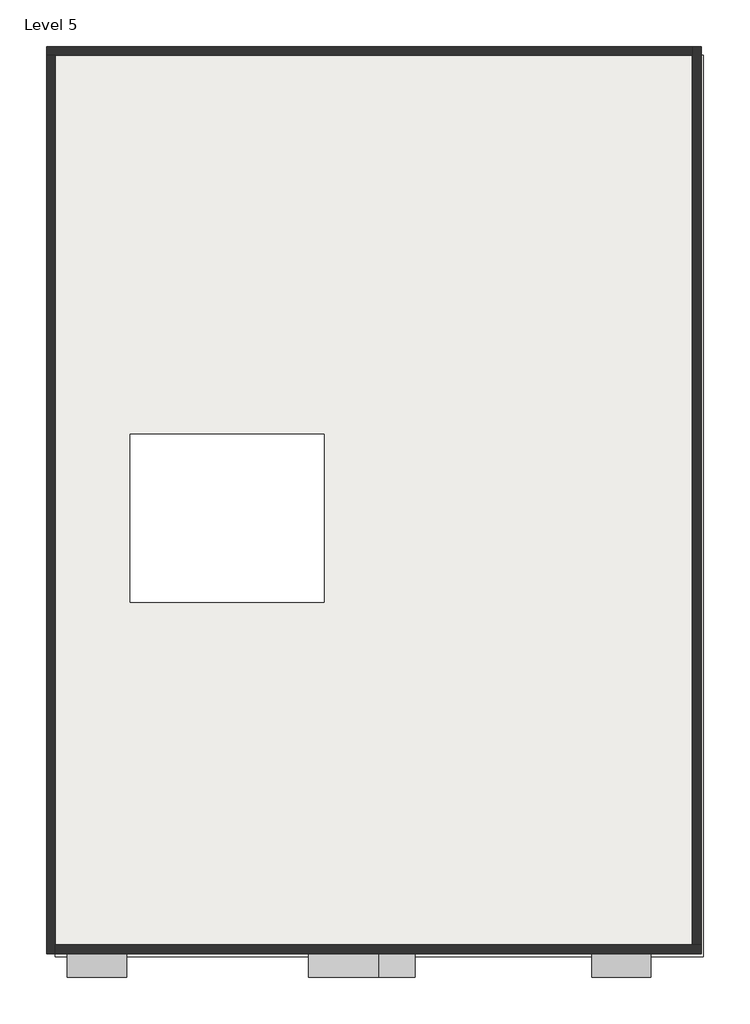
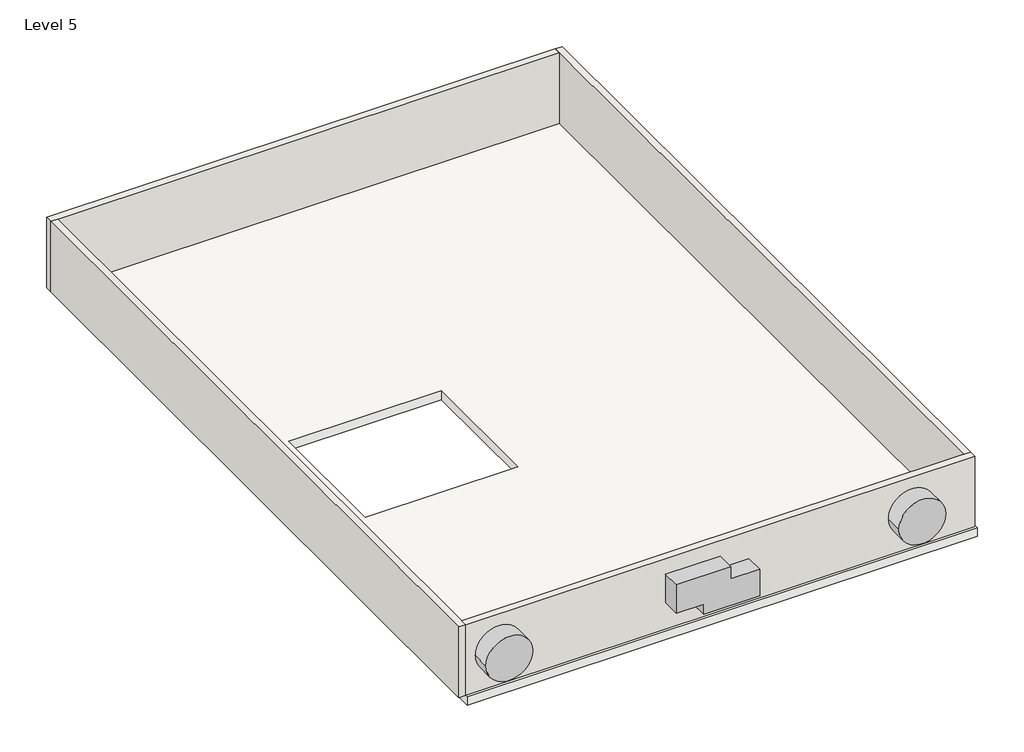
# One storey: 4 walls, 1 proxy, 1 roof.
"""IFC4 building model written with IfcOpenShell, lengths in millimetres."""

from ifc_helpers import new_model, si_unit, frame, origin, place, context, project, spatial, polyline, outline, extrude, faceted_brep, transform, mapped, element, save
from components import generic_models_1_generic_models_1_a3dca106

model = new_model("IFC4")

# Units and contexts
model_context = context("Model", 3, world=origin())
ifc_project = project(units=[si_unit("LENGTHUNIT", "METRE", prefix="MILLI")], contexts=[model_context])

# Site, building, storey
site = spatial("IfcSite", under=ifc_project)
building = spatial("IfcBuilding", under=site)
storey = spatial("IfcBuildingStorey", under=building, Name="Level 5", Elevation=9601.2)

# Proxy
placement = place(None, origin())
generic_models_1_generic_models_1_shape = generic_models_1_generic_models_1_a3dca106(model_context)
element("IfcBuildingElementProxy", 1, Name="Generic Models 1 : Generic Models 1", ObjectType="Generic Models 1 : Generic Models 1", at=placement, inside=storey, context=model_context, shape_type="MappedRepresentation", body=[
    mapped(generic_models_1_generic_models_1_shape, transform((0.0, 0.0, 0.0), x_axis=(1.0, 0.0, 0.0), y_axis=(0.0, 1.0, 0.0), z_axis=(0.0, 0.0, 1.0))),
])

# Roof
element("IfcRoof", 2, ObjectType="Generic - 12\"", at=placement, inside=storey, context=model_context, shape_type="SweptSolid", body=[
    extrude(outline(polyline([(-5216.1449167, -5813.0570853), (-5216.1449167, 5769.3429147), (3115.0550833, 5769.3429147), (3115.0550833, -5813.0570853), (-5216.1449167, -5813.0570853)]), holes=[polyline([(-1761.7449167, 898.8929147), (-4254.6766085, 898.8929147), (-4254.6766085, -1260.1070853), (-1761.7449167, -1260.1070853), (-1761.7449167, 898.8929147)])]), frame((0.0, 0.0, 9448.8), z_axis=(0.0, 0.0, 1.0), x_axis=(1.0, 0.0, 0.0)), (0.0, 0.0, 1.0), 152.4),
])

# Walls
element("IfcWall", 3, ObjectType="WALL4.5\"", at=placement, inside=storey, context=model_context, shape_type="Brep", body=[
    faceted_brep([(-5330.4449167, 5769.3429147, 9601.2), (-5216.1449167, 5769.3429147, 9601.2), (2975.3550833, 5769.3429147, 9601.2), (2975.3550833, 5769.3429147, 10820.4), (-5216.1449167, 5769.3429147, 10820.4), (-5330.4449167, 5769.3429147, 10820.4), (-5330.4449167, 5883.6429147, 9601.2), (-5330.4449167, 5883.6429147, 10820.4), (2975.3550833, 5883.6429147, 10820.4), (2975.3550833, 5883.6429147, 9601.2)], [[[0, 1, 2, 3, 4, 5]], [[6, 7, 8, 9]], [[2, 1, 0, 6, 9]], [[5, 4, 3, 8, 7]], [[0, 5, 7, 6]], [[3, 2, 9, 8]]]),
])
element("IfcWall", 4, ObjectType="WALL4.5\"", at=placement, inside=storey, context=model_context, shape_type="Brep", body=[
    faceted_brep([(-5216.1449167, -5774.9570853, 9601.2), (-5216.1449167, -5660.6570853, 9601.2), (-5216.1449167, 5769.3429147, 9601.2), (-5216.1449167, 5769.3429147, 10820.4), (-5216.1449167, -5660.6570853, 10820.4), (-5216.1449167, -5774.9570853, 10820.4), (-5330.4449167, -5774.9570853, 9601.2), (-5330.4449167, -5774.9570853, 10820.4), (-5330.4449167, 5769.3429147, 10820.4), (-5330.4449167, 5769.3429147, 9601.2)], [[[0, 1, 2, 3, 4, 5]], [[6, 7, 8, 9]], [[2, 1, 0, 6, 9]], [[5, 4, 3, 8, 7]], [[0, 5, 7, 6]], [[3, 2, 9, 8]]]),
])
element("IfcWall", 5, ObjectType="WALL4.5\"", at=placement, inside=storey, context=model_context, shape_type="Brep", body=[
    faceted_brep([(3089.6550833, -5660.6570853, 9601.2), (2975.3550833, -5660.6570853, 9601.2), (-5216.1449167, -5660.6570853, 9601.2), (-5216.1449167, -5660.6570853, 10820.4), (2975.3550833, -5660.6570853, 10820.4), (3089.6550833, -5660.6570853, 10820.4), (3089.6550833, -5774.9570853, 9601.2), (3089.6550833, -5774.9570853, 10820.4), (-5216.1449167, -5774.9570853, 10820.4), (-5216.1449167, -5774.9570853, 9601.2)], [[[0, 1, 2, 3, 4, 5]], [[6, 7, 8, 9]], [[2, 1, 0, 6, 9]], [[5, 4, 3, 8, 7]], [[0, 5, 7, 6]], [[3, 2, 9, 8]]]),
])
element("IfcWall", 6, ObjectType="WALL4.5\"", at=placement, inside=storey, context=model_context, shape_type="Brep", body=[
    faceted_brep([(2975.3550833, 5883.6429147, 9601.2), (2975.3550833, 5769.3429147, 9601.2), (2975.3550833, -5660.6570853, 9601.2), (2975.3550833, -5660.6570853, 10820.4), (2975.3550833, 5769.3429147, 10820.4), (2975.3550833, 5883.6429147, 10820.4), (3089.6550833, 5883.6429147, 9601.2), (3089.6550833, 5883.6429147, 10820.4), (3089.6550833, -5660.6570853, 10820.4), (3089.6550833, -5660.6570853, 9601.2)], [[[0, 1, 2, 3, 4, 5]], [[6, 7, 8, 9]], [[2, 1, 0, 6, 9]], [[5, 4, 3, 8, 7]], [[0, 5, 7, 6]], [[3, 2, 9, 8]]]),
])

save(model, "model.ifc")

# Revit data of these elements
# Type "Generic - 12\""
#   Assembly Code = "B1020"
#   Layers, outside or top first: 0' - 6" no material (function 1)
# Type "WALL4.5\""
#   Assembly Code = "B2010"
#   Layers, outside or top first: 0' - 4 1/2" no material (function 1)
# Element 1 (IfcBuildingElementProxy, "Generic Models 1 : Generic Models 1")
#   Phase Created = New Construction
#   Materials on its faces: "Parking Stripe"
# Element 2 (IfcRoof, "Generic - 12\"")
#   built-in parameter 1001705 = 31.5 (stored number, unit not read)
#   built-in parameter 1001701 = -0.5 (stored number, unit not read)
#   built-in parameter 1001710 = 33615
#   Phase Created = New Construction
#   Materials on its faces: "Default Roof"
# Elements 3, 4, 5, 6 (IfcWall, "WALL4.5\"")
#   Top Offset = 0' - 0"
#   Base Offset = 0' - 0"
#   Unconnected Height = 4' - 0"
#   wall height = 4' - 0"
#   Phase Created = New Construction
#   Base Constraint = Level 5
#   Materials on its faces: "Default Wall", "Door - Frame"
# Materials
#   "Parking Stripe": class "Paint", colour RGB 250 250 91, transparency 0, Cost = 0
#   "Default Roof": colour RGB 88 101 114, transparency 0, Cost = 0
#   "Default Wall": colour RGB 128 128 128, transparency 0, Cost = 0
#   "Door - Frame": colour RGB 118 70 51, transparency 0, Cost = 0
